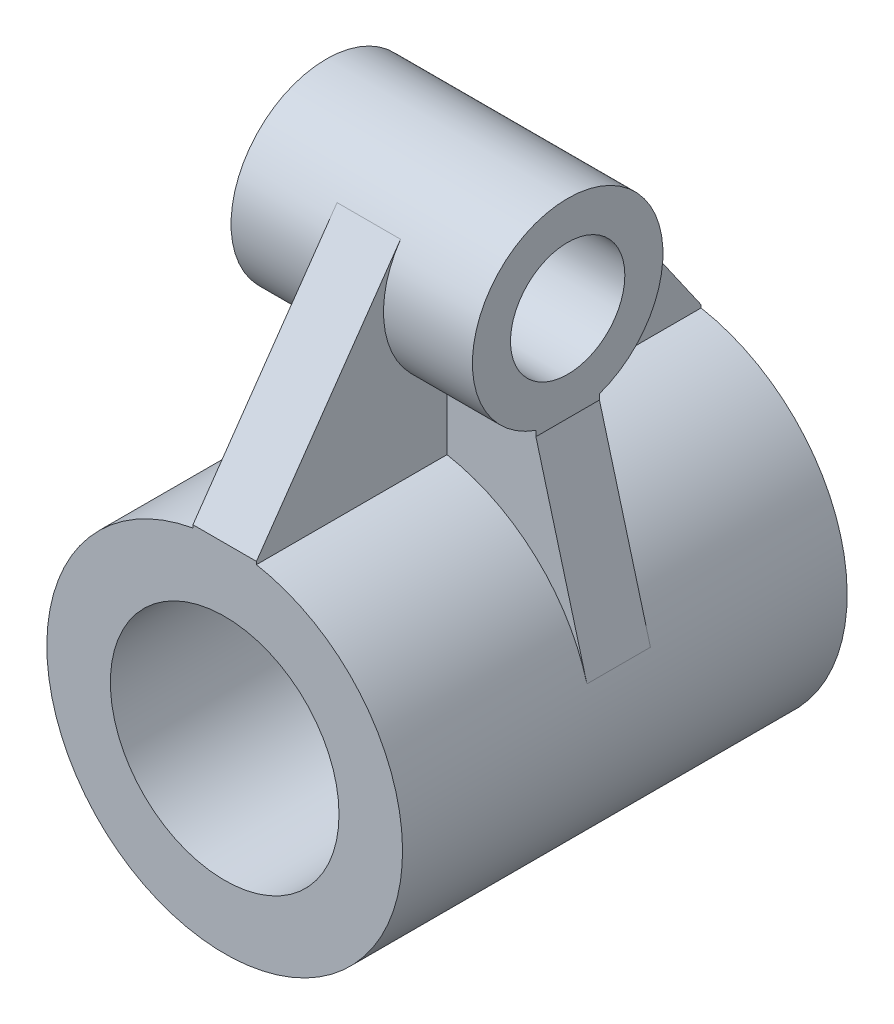
ISO-10303-21;
HEADER;
FILE_DESCRIPTION(('STEP AP214'),'2;1');
FILE_NAME('part.step','',(''),(''),'','','');
FILE_SCHEMA(('AUTOMOTIVE_DESIGN { 1 0 10303 214 1 1 1 1 }'));
ENDSEC;
DATA;
#1=APPLICATION_CONTEXT('core data for automotive mechanical design processes');
#2=APPLICATION_PROTOCOL_DEFINITION('international standard','automotive_design',2000,#1);
#3=PRODUCT_CONTEXT('',#1,'mechanical');
#4=PRODUCT('Part','Part','',(#3));
#5=PRODUCT_RELATED_PRODUCT_CATEGORY('part','',(#4));
#6=PRODUCT_DEFINITION_FORMATION('','',#4);
#7=PRODUCT_DEFINITION_CONTEXT('part definition',#1,'design');
#8=PRODUCT_DEFINITION('design','',#6,#7);
#9=PRODUCT_DEFINITION_SHAPE('','',#8);
#10=(LENGTH_UNIT() NAMED_UNIT(*) SI_UNIT(.MILLI.,.METRE.));
#11=(NAMED_UNIT(*) PLANE_ANGLE_UNIT() SI_UNIT($,.RADIAN.));
#12=(NAMED_UNIT(*) SI_UNIT($,.STERADIAN.) SOLID_ANGLE_UNIT());
#13=UNCERTAINTY_MEASURE_WITH_UNIT(LENGTH_MEASURE(1.E-05),#10,'distance_accuracy_value','');
#14=(GEOMETRIC_REPRESENTATION_CONTEXT(3) GLOBAL_UNCERTAINTY_ASSIGNED_CONTEXT((#13)) GLOBAL_UNIT_ASSIGNED_CONTEXT((#10,
#11,#12)) REPRESENTATION_CONTEXT('',''));
#15=CARTESIAN_POINT('',(0.,0.,0.));
#16=DIRECTION('',(0.,0.,1.));
#17=DIRECTION('',(1.,0.,0.));
#18=AXIS2_PLACEMENT_3D('',#15,#16,#17);
#19=CARTESIAN_POINT('',(0.,0.,17.5));
#20=DIRECTION('',(0.,0.,-1.));
#21=DIRECTION('',(-1.,0.,0.));
#22=AXIS2_PLACEMENT_3D('',#19,#20,#21);
#23=CYLINDRICAL_SURFACE('',#22,14.);
#24=CARTESIAN_POINT('',(0.,0.,2.5));
#25=DIRECTION('',(0.,0.,-1.));
#26=DIRECTION('',(1.,0.,0.));
#27=AXIS2_PLACEMENT_3D('',#24,#25,#26);
#28=CIRCLE('',#27,14.);
#29=CARTESIAN_POINT('',(-13.5145575336428,3.65468667191318,2.5));
#30=VERTEX_POINT('',#29);
#31=CARTESIAN_POINT('',(-2.5,13.7749773139559,2.5));
#32=VERTEX_POINT('',#31);
#33=EDGE_CURVE('E182',#30,#32,#28,.T.);
#34=ORIENTED_EDGE('',*,*,#33,.F.);
#35=DIRECTION('',(0.,0.,-1.));
#36=VECTOR('',#35,1.);
#37=CARTESIAN_POINT('',(-13.5145575336428,3.65468667191318,2.5));
#38=LINE('',#37,#36);
#39=CARTESIAN_POINT('',(-13.5145575336428,3.65468667191318,-2.5));
#40=VERTEX_POINT('',#39);
#41=EDGE_CURVE('E178',#30,#40,#38,.T.);
#42=ORIENTED_EDGE('',*,*,#41,.T.);
#43=CARTESIAN_POINT('',(0.,0.,-2.5));
#44=DIRECTION('',(0.,0.,-1.));
#45=DIRECTION('',(1.,0.,0.));
#46=AXIS2_PLACEMENT_3D('',#43,#44,#45);
#47=CIRCLE('',#46,14.);
#48=CARTESIAN_POINT('',(-2.5,13.7749773139559,-2.5));
#49=VERTEX_POINT('',#48);
#50=EDGE_CURVE('E190',#40,#49,#47,.T.);
#51=ORIENTED_EDGE('',*,*,#50,.T.);
#52=DIRECTION('',(0.,0.,-1.));
#53=VECTOR('',#52,1.);
#54=CARTESIAN_POINT('',(-2.5,13.7749773139559,17.5));
#55=LINE('',#54,#53);
#56=CARTESIAN_POINT('',(-2.5,13.7749773139559,-17.5));
#57=VERTEX_POINT('',#56);
#58=EDGE_CURVE('E11',#57,#49,#55,.F.);
#59=ORIENTED_EDGE('',*,*,#58,.F.);
#60=CARTESIAN_POINT('',(0.,0.,-17.5));
#61=DIRECTION('',(0.,0.,1.));
#62=DIRECTION('',(1.,0.,0.));
#63=AXIS2_PLACEMENT_3D('',#60,#61,#62);
#64=CIRCLE('',#63,14.);
#65=CARTESIAN_POINT('',(2.5,13.7749773139559,-17.5));
#66=VERTEX_POINT('',#65);
#67=EDGE_CURVE('E272',#57,#66,#64,.T.);
#68=ORIENTED_EDGE('',*,*,#67,.T.);
#69=DIRECTION('',(0.,0.,-1.));
#70=VECTOR('',#69,1.);
#71=CARTESIAN_POINT('',(2.5,13.7749773139559,17.5));
#72=LINE('',#71,#70);
#73=CARTESIAN_POINT('',(2.5,13.7749773139559,-2.5));
#74=VERTEX_POINT('',#73);
#75=EDGE_CURVE('E280',#74,#66,#72,.T.);
#76=ORIENTED_EDGE('',*,*,#75,.F.);
#77=CARTESIAN_POINT('',(13.5145575336428,3.65468667191318,-2.5));
#78=VERTEX_POINT('',#77);
#79=EDGE_CURVE('E59',#74,#78,#47,.T.);
#80=ORIENTED_EDGE('',*,*,#79,.T.);
#81=DIRECTION('',(0.,0.,-1.));
#82=VECTOR('',#81,1.);
#83=CARTESIAN_POINT('',(13.5145575336428,3.65468667191318,2.5));
#84=LINE('',#83,#82);
#85=CARTESIAN_POINT('',(13.5145575336428,3.65468667191318,2.5));
#86=VERTEX_POINT('',#85);
#87=EDGE_CURVE('E52',#86,#78,#84,.T.);
#88=ORIENTED_EDGE('',*,*,#87,.F.);
#89=CARTESIAN_POINT('',(2.5,13.7749773139559,2.5));
#90=VERTEX_POINT('',#89);
#91=EDGE_CURVE('E191',#90,#86,#28,.T.);
#92=ORIENTED_EDGE('',*,*,#91,.F.);
#93=CARTESIAN_POINT('',(2.5,13.7749773139559,17.5));
#94=VERTEX_POINT('',#93);
#95=EDGE_CURVE('E276',#94,#90,#72,.T.);
#96=ORIENTED_EDGE('',*,*,#95,.F.);
#97=CARTESIAN_POINT('',(0.,0.,17.5));
#98=DIRECTION('',(0.,0.,1.));
#99=DIRECTION('',(1.,0.,0.));
#100=AXIS2_PLACEMENT_3D('',#97,#98,#99);
#101=CIRCLE('',#100,14.);
#102=CARTESIAN_POINT('',(-2.5,13.7749773139559,17.5));
#103=VERTEX_POINT('',#102);
#104=EDGE_CURVE('E274',#103,#94,#101,.T.);
#105=ORIENTED_EDGE('',*,*,#104,.F.);
#106=EDGE_CURVE('E46',#32,#103,#55,.F.);
#107=ORIENTED_EDGE('',*,*,#106,.F.);
#108=EDGE_LOOP('',(#34,#42,#51,#59,#68,#76,#80,#88,#92,#96,#105,#107));
#109=FACE_BOUND('',#108,.T.);
#110=ADVANCED_FACE('F39',(#109),#23,.T.);
#111=CARTESIAN_POINT('',(-2.5,11.,17.5));
#112=DIRECTION('',(1.,0.,0.));
#113=DIRECTION('',(0.,0.,-1.));
#114=AXIS2_PLACEMENT_3D('',#111,#112,#113);
#115=PLANE('',#114);
#116=ORIENTED_EDGE('',*,*,#58,.T.);
#117=DIRECTION('',(0.,-1.,0.));
#118=VECTOR('',#117,1.);
#119=CARTESIAN_POINT('',(-2.5,26.,-2.5));
#120=LINE('',#119,#118);
#121=CARTESIAN_POINT('',(-2.5,18.9289321881345,-2.5));
#122=VERTEX_POINT('',#121);
#123=EDGE_CURVE('E243',#122,#49,#120,.T.);
#124=ORIENTED_EDGE('',*,*,#123,.F.);
#125=CARTESIAN_POINT('',(-2.5,26.,0.));
#126=DIRECTION('',(-1.,0.,0.));
#127=DIRECTION('',(0.,0.,-1.));
#128=AXIS2_PLACEMENT_3D('',#125,#126,#127);
#129=CIRCLE('',#128,7.5);
#130=CARTESIAN_POINT('',(-2.5,30.2870363418498,-6.15396777726847));
#131=VERTEX_POINT('',#130);
#132=EDGE_CURVE('E223',#131,#122,#129,.T.);
#133=ORIENTED_EDGE('',*,*,#132,.F.);
#134=DIRECTION('',(0.,0.820529036969129,0.57160484557998));
#135=VECTOR('',#134,1.);
#136=CARTESIAN_POINT('',(-2.5,14.,-17.5));
#137=LINE('',#136,#135);
#138=CARTESIAN_POINT('',(-2.5,14.,-17.5));
#139=VERTEX_POINT('',#138);
#140=EDGE_CURVE('E219',#139,#131,#137,.T.);
#141=ORIENTED_EDGE('',*,*,#140,.F.);
#142=DIRECTION('',(0.,1.,0.));
#143=VECTOR('',#142,1.);
#144=CARTESIAN_POINT('',(-2.5,11.,-17.5));
#145=LINE('',#144,#143);
#146=EDGE_CURVE('E264',#57,#139,#145,.T.);
#147=ORIENTED_EDGE('',*,*,#146,.F.);
#148=EDGE_LOOP('',(#116,#124,#133,#141,#147));
#149=FACE_BOUND('',#148,.T.);
#150=ADVANCED_FACE('F350',(#149),#115,.F.);
#151=DIRECTION('',(0.,1.,0.));
#152=VECTOR('',#151,1.);
#153=CARTESIAN_POINT('',(-2.5,11.,2.5));
#154=LINE('',#153,#152);
#155=CARTESIAN_POINT('',(-2.5,18.9289321881345,2.5));
#156=VERTEX_POINT('',#155);
#157=EDGE_CURVE('E252',#32,#156,#154,.T.);
#158=ORIENTED_EDGE('',*,*,#157,.F.);
#159=ORIENTED_EDGE('',*,*,#106,.T.);
#160=DIRECTION('',(0.,1.,0.));
#161=VECTOR('',#160,1.);
#162=CARTESIAN_POINT('',(-2.5,11.,17.5));
#163=LINE('',#162,#161);
#164=CARTESIAN_POINT('',(-2.5,14.,17.5));
#165=VERTEX_POINT('',#164);
#166=EDGE_CURVE('E259',#103,#165,#163,.T.);
#167=ORIENTED_EDGE('',*,*,#166,.T.);
#168=DIRECTION('',(0.,-0.820529036969129,0.57160484557998));
#169=VECTOR('',#168,1.);
#170=CARTESIAN_POINT('',(-2.5,14.,17.5));
#171=LINE('',#170,#169);
#172=CARTESIAN_POINT('',(-2.5,30.2870363418499,6.15396777726847));
#173=VERTEX_POINT('',#172);
#174=EDGE_CURVE('E215',#173,#165,#171,.T.);
#175=ORIENTED_EDGE('',*,*,#174,.F.);
#176=EDGE_CURVE('E225',#156,#173,#129,.T.);
#177=ORIENTED_EDGE('',*,*,#176,.F.);
#178=EDGE_LOOP('',(#158,#159,#167,#175,#177));
#179=FACE_BOUND('',#178,.T.);
#180=ADVANCED_FACE('F316',(#179),#115,.F.);
#181=CARTESIAN_POINT('',(2.5,11.,17.5));
#182=DIRECTION('',(-1.,0.,0.));
#183=DIRECTION('',(0.,0.,1.));
#184=AXIS2_PLACEMENT_3D('',#181,#182,#183);
#185=PLANE('',#184);
#186=DIRECTION('',(0.,-1.,0.));
#187=VECTOR('',#186,1.);
#188=CARTESIAN_POINT('',(2.5,11.,2.5));
#189=LINE('',#188,#187);
#190=CARTESIAN_POINT('',(2.5,18.9289321881345,2.5));
#191=VERTEX_POINT('',#190);
#192=EDGE_CURVE('E247',#191,#90,#189,.T.);
#193=ORIENTED_EDGE('',*,*,#192,.F.);
#194=CARTESIAN_POINT('',(2.5,26.,0.));
#195=DIRECTION('',(-1.,0.,0.));
#196=DIRECTION('',(0.,0.,-1.));
#197=AXIS2_PLACEMENT_3D('',#194,#195,#196);
#198=CIRCLE('',#197,7.5);
#199=CARTESIAN_POINT('',(2.5,30.2870363418499,6.15396777726847));
#200=VERTEX_POINT('',#199);
#201=EDGE_CURVE('E212',#191,#200,#198,.T.);
#202=ORIENTED_EDGE('',*,*,#201,.T.);
#203=DIRECTION('',(0.,-0.820529036969129,0.57160484557998));
#204=VECTOR('',#203,1.);
#205=CARTESIAN_POINT('',(2.5,14.,17.5));
#206=LINE('',#205,#204);
#207=CARTESIAN_POINT('',(2.5,14.,17.5));
#208=VERTEX_POINT('',#207);
#209=EDGE_CURVE('E216',#200,#208,#206,.T.);
#210=ORIENTED_EDGE('',*,*,#209,.T.);
#211=DIRECTION('',(0.,1.,0.));
#212=VECTOR('',#211,1.);
#213=CARTESIAN_POINT('',(2.5,11.,17.5));
#214=LINE('',#213,#212);
#215=EDGE_CURVE('E261',#94,#208,#214,.T.);
#216=ORIENTED_EDGE('',*,*,#215,.F.);
#217=ORIENTED_EDGE('',*,*,#95,.T.);
#218=EDGE_LOOP('',(#193,#202,#210,#216,#217));
#219=FACE_BOUND('',#218,.T.);
#220=ADVANCED_FACE('F328',(#219),#185,.F.);
#221=DIRECTION('',(0.,1.,0.));
#222=VECTOR('',#221,1.);
#223=CARTESIAN_POINT('',(2.5,11.,-2.5));
#224=LINE('',#223,#222);
#225=CARTESIAN_POINT('',(2.5,18.9289321881345,-2.5));
#226=VERTEX_POINT('',#225);
#227=EDGE_CURVE('E246',#74,#226,#224,.T.);
#228=ORIENTED_EDGE('',*,*,#227,.F.);
#229=ORIENTED_EDGE('',*,*,#75,.T.);
#230=DIRECTION('',(0.,1.,0.));
#231=VECTOR('',#230,1.);
#232=CARTESIAN_POINT('',(2.5,11.,-17.5));
#233=LINE('',#232,#231);
#234=CARTESIAN_POINT('',(2.5,14.,-17.5));
#235=VERTEX_POINT('',#234);
#236=EDGE_CURVE('E263',#66,#235,#233,.T.);
#237=ORIENTED_EDGE('',*,*,#236,.T.);
#238=DIRECTION('',(0.,0.820529036969129,0.57160484557998));
#239=VECTOR('',#238,1.);
#240=CARTESIAN_POINT('',(2.5,14.,-17.5));
#241=LINE('',#240,#239);
#242=CARTESIAN_POINT('',(2.5,30.2870363418498,-6.15396777726847));
#243=VERTEX_POINT('',#242);
#244=EDGE_CURVE('E206',#235,#243,#241,.T.);
#245=ORIENTED_EDGE('',*,*,#244,.T.);
#246=EDGE_CURVE('E214',#243,#226,#198,.T.);
#247=ORIENTED_EDGE('',*,*,#246,.T.);
#248=EDGE_LOOP('',(#228,#229,#237,#245,#247));
#249=FACE_BOUND('',#248,.T.);
#250=ADVANCED_FACE('F282',(#249),#185,.F.);
#251=CARTESIAN_POINT('',(0.,0.,17.5));
#252=DIRECTION('',(0.,0.,1.));
#253=DIRECTION('',(1.,0.,0.));
#254=AXIS2_PLACEMENT_3D('',#251,#252,#253);
#255=PLANE('',#254);
#256=ORIENTED_EDGE('',*,*,#104,.T.);
#257=ORIENTED_EDGE('',*,*,#215,.T.);
#258=DIRECTION('',(-1.,0.,0.));
#259=VECTOR('',#258,1.);
#260=CARTESIAN_POINT('',(-2.5,14.,17.5));
#261=LINE('',#260,#259);
#262=EDGE_CURVE('E257',#208,#165,#261,.T.);
#263=ORIENTED_EDGE('',*,*,#262,.T.);
#264=ORIENTED_EDGE('',*,*,#166,.F.);
#265=EDGE_LOOP('',(#256,#257,#263,#264));
#266=FACE_BOUND('',#265,.T.);
#267=CARTESIAN_POINT('',(0.,0.,17.5));
#268=DIRECTION('',(0.,0.,1.));
#269=DIRECTION('',(1.,0.,0.));
#270=AXIS2_PLACEMENT_3D('',#267,#268,#269);
#271=CIRCLE('',#270,9.);
#272=CARTESIAN_POINT('',(9.,0.,17.5));
#273=VERTEX_POINT('',#272);
#274=EDGE_CURVE('E270',#273,#273,#271,.T.);
#275=ORIENTED_EDGE('',*,*,#274,.F.);
#276=EDGE_LOOP('',(#275));
#277=FACE_BOUND('',#276,.T.);
#278=ADVANCED_FACE('F329',(#266,#277),#255,.T.);
#279=CARTESIAN_POINT('',(0.,0.,-17.5));
#280=DIRECTION('',(0.,0.,1.));
#281=DIRECTION('',(1.,0.,0.));
#282=AXIS2_PLACEMENT_3D('',#279,#280,#281);
#283=PLANE('',#282);
#284=ORIENTED_EDGE('',*,*,#146,.T.);
#285=DIRECTION('',(1.,0.,0.));
#286=VECTOR('',#285,1.);
#287=CARTESIAN_POINT('',(-2.5,14.,-17.5));
#288=LINE('',#287,#286);
#289=EDGE_CURVE('E254',#139,#235,#288,.T.);
#290=ORIENTED_EDGE('',*,*,#289,.T.);
#291=ORIENTED_EDGE('',*,*,#236,.F.);
#292=ORIENTED_EDGE('',*,*,#67,.F.);
#293=EDGE_LOOP('',(#284,#290,#291,#292));
#294=FACE_BOUND('',#293,.T.);
#295=CARTESIAN_POINT('',(0.,0.,-17.5));
#296=DIRECTION('',(0.,0.,1.));
#297=DIRECTION('',(1.,0.,0.));
#298=AXIS2_PLACEMENT_3D('',#295,#296,#297);
#299=CIRCLE('',#298,9.);
#300=CARTESIAN_POINT('',(9.,0.,-17.5));
#301=VERTEX_POINT('',#300);
#302=EDGE_CURVE('E266',#301,#301,#299,.T.);
#303=ORIENTED_EDGE('',*,*,#302,.T.);
#304=EDGE_LOOP('',(#303));
#305=FACE_BOUND('',#304,.T.);
#306=ADVANCED_FACE('F288',(#294,#305),#283,.F.);
#307=CARTESIAN_POINT('',(0.,0.,17.5));
#308=DIRECTION('',(0.,0.,-1.));
#309=DIRECTION('',(-1.,0.,0.));
#310=AXIS2_PLACEMENT_3D('',#307,#308,#309);
#311=CYLINDRICAL_SURFACE('',#310,9.);
#312=ORIENTED_EDGE('',*,*,#274,.T.);
#313=EDGE_LOOP('',(#312));
#314=FACE_BOUND('',#313,.T.);
#315=ORIENTED_EDGE('',*,*,#302,.F.);
#316=EDGE_LOOP('',(#315));
#317=FACE_BOUND('',#316,.T.);
#318=ADVANCED_FACE('F337',(#314,#317),#311,.F.);
#319=CARTESIAN_POINT('',(-9.5,21.5,-2.5));
#320=DIRECTION('',(0.,0.,1.));
#321=DIRECTION('',(1.,0.,0.));
#322=AXIS2_PLACEMENT_3D('',#319,#320,#321);
#323=PLANE('',#322);
#324=ORIENTED_EDGE('',*,*,#123,.T.);
#325=ORIENTED_EDGE('',*,*,#50,.F.);
#326=DIRECTION('',(-0.261049047993799,-0.96532553811734,0.));
#327=VECTOR('',#326,1.);
#328=CARTESIAN_POINT('',(-13.5145575336428,3.65468667191318,-2.5));
#329=LINE('',#328,#327);
#330=CARTESIAN_POINT('',(-9.5,18.5,-2.5));
#331=VERTEX_POINT('',#330);
#332=EDGE_CURVE('E194',#331,#40,#329,.T.);
#333=ORIENTED_EDGE('',*,*,#332,.F.);
#334=DIRECTION('',(0.,-1.,0.));
#335=VECTOR('',#334,1.);
#336=CARTESIAN_POINT('',(-9.5,21.5,-2.5));
#337=LINE('',#336,#335);
#338=CARTESIAN_POINT('',(-9.5,18.9289321881345,-2.5));
#339=VERTEX_POINT('',#338);
#340=EDGE_CURVE('E171',#339,#331,#337,.T.);
#341=ORIENTED_EDGE('',*,*,#340,.F.);
#342=DIRECTION('',(-1.,0.,0.));
#343=VECTOR('',#342,1.);
#344=CARTESIAN_POINT('',(9.5,18.9289321881345,-2.5));
#345=LINE('',#344,#343);
#346=EDGE_CURVE('E161',#339,#122,#345,.F.);
#347=ORIENTED_EDGE('',*,*,#346,.T.);
#348=EDGE_LOOP('',(#324,#325,#333,#341,#347));
#349=FACE_BOUND('',#348,.T.);
#350=ADVANCED_FACE('F339',(#349),#323,.F.);
#351=CARTESIAN_POINT('',(-9.5,21.5,2.5));
#352=DIRECTION('',(0.,0.,-1.));
#353=DIRECTION('',(-1.,0.,0.));
#354=AXIS2_PLACEMENT_3D('',#351,#352,#353);
#355=PLANE('',#354);
#356=ORIENTED_EDGE('',*,*,#33,.T.);
#357=ORIENTED_EDGE('',*,*,#157,.T.);
#358=DIRECTION('',(-1.,0.,0.));
#359=VECTOR('',#358,1.);
#360=CARTESIAN_POINT('',(9.5,18.9289321881345,2.5));
#361=LINE('',#360,#359);
#362=CARTESIAN_POINT('',(-9.5,18.9289321881345,2.5));
#363=VERTEX_POINT('',#362);
#364=EDGE_CURVE('E157',#156,#363,#361,.T.);
#365=ORIENTED_EDGE('',*,*,#364,.T.);
#366=DIRECTION('',(0.,-1.,0.));
#367=VECTOR('',#366,1.);
#368=CARTESIAN_POINT('',(-9.5,21.5,2.5));
#369=LINE('',#368,#367);
#370=CARTESIAN_POINT('',(-9.5,18.5,2.5));
#371=VERTEX_POINT('',#370);
#372=EDGE_CURVE('E155',#363,#371,#369,.T.);
#373=ORIENTED_EDGE('',*,*,#372,.T.);
#374=DIRECTION('',(-0.261049047993799,-0.96532553811734,0.));
#375=VECTOR('',#374,1.);
#376=CARTESIAN_POINT('',(-13.5145575336428,3.65468667191318,2.5));
#377=LINE('',#376,#375);
#378=EDGE_CURVE('E156',#371,#30,#377,.T.);
#379=ORIENTED_EDGE('',*,*,#378,.T.);
#380=EDGE_LOOP('',(#356,#357,#365,#373,#379));
#381=FACE_BOUND('',#380,.T.);
#382=ADVANCED_FACE('F154',(#381),#355,.F.);
#383=CARTESIAN_POINT('',(9.5,18.9289321881345,2.5));
#384=VERTEX_POINT('',#383);
#385=EDGE_CURVE('E210',#384,#191,#361,.T.);
#386=ORIENTED_EDGE('',*,*,#385,.T.);
#387=ORIENTED_EDGE('',*,*,#192,.T.);
#388=ORIENTED_EDGE('',*,*,#91,.T.);
#389=DIRECTION('',(-0.261049047993799,0.96532553811734,0.));
#390=VECTOR('',#389,1.);
#391=CARTESIAN_POINT('',(9.5,18.5,2.5));
#392=LINE('',#391,#390);
#393=CARTESIAN_POINT('',(9.5,18.5,2.5));
#394=VERTEX_POINT('',#393);
#395=EDGE_CURVE('E177',#86,#394,#392,.T.);
#396=ORIENTED_EDGE('',*,*,#395,.T.);
#397=DIRECTION('',(0.,-1.,0.));
#398=VECTOR('',#397,1.);
#399=CARTESIAN_POINT('',(9.5,21.5,2.5));
#400=LINE('',#399,#398);
#401=EDGE_CURVE('E165',#384,#394,#400,.T.);
#402=ORIENTED_EDGE('',*,*,#401,.F.);
#403=EDGE_LOOP('',(#386,#387,#388,#396,#402));
#404=FACE_BOUND('',#403,.T.);
#405=ADVANCED_FACE('F313',(#404),#355,.F.);
#406=ORIENTED_EDGE('',*,*,#79,.F.);
#407=ORIENTED_EDGE('',*,*,#227,.T.);
#408=CARTESIAN_POINT('',(9.5,18.9289321881345,-2.5));
#409=VERTEX_POINT('',#408);
#410=EDGE_CURVE('E202',#226,#409,#345,.F.);
#411=ORIENTED_EDGE('',*,*,#410,.T.);
#412=DIRECTION('',(0.,-1.,0.));
#413=VECTOR('',#412,1.);
#414=CARTESIAN_POINT('',(9.5,21.5,-2.5));
#415=LINE('',#414,#413);
#416=CARTESIAN_POINT('',(9.5,18.5,-2.5));
#417=VERTEX_POINT('',#416);
#418=EDGE_CURVE('E197',#409,#417,#415,.T.);
#419=ORIENTED_EDGE('',*,*,#418,.T.);
#420=DIRECTION('',(-0.261049047993799,0.96532553811734,0.));
#421=VECTOR('',#420,1.);
#422=CARTESIAN_POINT('',(9.5,18.5,-2.5));
#423=LINE('',#422,#421);
#424=EDGE_CURVE('E188',#78,#417,#423,.T.);
#425=ORIENTED_EDGE('',*,*,#424,.F.);
#426=EDGE_LOOP('',(#406,#407,#411,#419,#425));
#427=FACE_BOUND('',#426,.T.);
#428=ADVANCED_FACE('F302',(#427),#323,.F.);
#429=CARTESIAN_POINT('',(9.5,26.,0.));
#430=DIRECTION('',(-1.,0.,0.));
#431=DIRECTION('',(0.,0.,1.));
#432=AXIS2_PLACEMENT_3D('',#429,#430,#431);
#433=CYLINDRICAL_SURFACE('',#432,7.5);
#434=ORIENTED_EDGE('',*,*,#385,.F.);
#435=CARTESIAN_POINT('',(9.5,26.,0.));
#436=DIRECTION('',(1.,0.,0.));
#437=DIRECTION('',(0.,0.,-1.));
#438=AXIS2_PLACEMENT_3D('',#435,#436,#437);
#439=CIRCLE('',#438,7.5);
#440=EDGE_CURVE('E239',#409,#384,#439,.T.);
#441=ORIENTED_EDGE('',*,*,#440,.F.);
#442=ORIENTED_EDGE('',*,*,#410,.F.);
#443=ORIENTED_EDGE('',*,*,#246,.F.);
#444=DIRECTION('',(-1.,0.,0.));
#445=VECTOR('',#444,1.);
#446=CARTESIAN_POINT('',(2.5,30.2870363418498,-6.15396777726847));
#447=LINE('',#446,#445);
#448=EDGE_CURVE('E233',#243,#131,#447,.T.);
#449=ORIENTED_EDGE('',*,*,#448,.T.);
#450=ORIENTED_EDGE('',*,*,#132,.T.);
#451=ORIENTED_EDGE('',*,*,#346,.F.);
#452=CARTESIAN_POINT('',(-9.5,26.,0.));
#453=DIRECTION('',(1.,0.,0.));
#454=DIRECTION('',(0.,0.,-1.));
#455=AXIS2_PLACEMENT_3D('',#452,#453,#454);
#456=CIRCLE('',#455,7.5);
#457=EDGE_CURVE('E240',#339,#363,#456,.T.);
#458=ORIENTED_EDGE('',*,*,#457,.T.);
#459=ORIENTED_EDGE('',*,*,#364,.F.);
#460=ORIENTED_EDGE('',*,*,#176,.T.);
#461=DIRECTION('',(-1.,0.,0.));
#462=VECTOR('',#461,1.);
#463=CARTESIAN_POINT('',(2.5,30.2870363418499,6.15396777726847));
#464=LINE('',#463,#462);
#465=EDGE_CURVE('E217',#200,#173,#464,.T.);
#466=ORIENTED_EDGE('',*,*,#465,.F.);
#467=ORIENTED_EDGE('',*,*,#201,.F.);
#468=EDGE_LOOP('',(#434,#441,#442,#443,#449,#450,#451,#458,#459,#460,#466,#467));
#469=FACE_BOUND('',#468,.T.);
#470=ADVANCED_FACE('F297',(#469),#433,.T.);
#471=CARTESIAN_POINT('',(9.5,26.,0.));
#472=DIRECTION('',(1.,0.,0.));
#473=DIRECTION('',(0.,0.,-1.));
#474=AXIS2_PLACEMENT_3D('',#471,#472,#473);
#475=PLANE('',#474);
#476=ORIENTED_EDGE('',*,*,#440,.T.);
#477=ORIENTED_EDGE('',*,*,#401,.T.);
#478=DIRECTION('',(0.,0.,-1.));
#479=VECTOR('',#478,1.);
#480=CARTESIAN_POINT('',(9.5,18.5,-2.5));
#481=LINE('',#480,#479);
#482=EDGE_CURVE('E174',#394,#417,#481,.T.);
#483=ORIENTED_EDGE('',*,*,#482,.T.);
#484=ORIENTED_EDGE('',*,*,#418,.F.);
#485=EDGE_LOOP('',(#476,#477,#483,#484));
#486=FACE_BOUND('',#485,.T.);
#487=CARTESIAN_POINT('',(9.5,26.,0.));
#488=DIRECTION('',(1.,0.,0.));
#489=DIRECTION('',(0.,0.,-1.));
#490=AXIS2_PLACEMENT_3D('',#487,#488,#489);
#491=CIRCLE('',#490,4.5);
#492=CARTESIAN_POINT('',(9.5,26.,-4.5));
#493=VERTEX_POINT('',#492);
#494=EDGE_CURVE('E234',#493,#493,#491,.T.);
#495=ORIENTED_EDGE('',*,*,#494,.F.);
#496=EDGE_LOOP('',(#495));
#497=FACE_BOUND('',#496,.T.);
#498=ADVANCED_FACE('F306',(#486,#497),#475,.T.);
#499=CARTESIAN_POINT('',(-9.5,26.,0.));
#500=DIRECTION('',(1.,0.,0.));
#501=DIRECTION('',(0.,0.,-1.));
#502=AXIS2_PLACEMENT_3D('',#499,#500,#501);
#503=PLANE('',#502);
#504=ORIENTED_EDGE('',*,*,#340,.T.);
#505=DIRECTION('',(0.,0.,1.));
#506=VECTOR('',#505,1.);
#507=CARTESIAN_POINT('',(-9.5,18.5,-2.5));
#508=LINE('',#507,#506);
#509=EDGE_CURVE('E170',#331,#371,#508,.T.);
#510=ORIENTED_EDGE('',*,*,#509,.T.);
#511=ORIENTED_EDGE('',*,*,#372,.F.);
#512=ORIENTED_EDGE('',*,*,#457,.F.);
#513=EDGE_LOOP('',(#504,#510,#511,#512));
#514=FACE_BOUND('',#513,.T.);
#515=CARTESIAN_POINT('',(-9.5,26.,0.));
#516=DIRECTION('',(1.,0.,0.));
#517=DIRECTION('',(0.,0.,-1.));
#518=AXIS2_PLACEMENT_3D('',#515,#516,#517);
#519=CIRCLE('',#518,4.5);
#520=CARTESIAN_POINT('',(-9.5,26.,-4.5));
#521=VERTEX_POINT('',#520);
#522=EDGE_CURVE('E231',#521,#521,#519,.T.);
#523=ORIENTED_EDGE('',*,*,#522,.T.);
#524=EDGE_LOOP('',(#523));
#525=FACE_BOUND('',#524,.T.);
#526=ADVANCED_FACE('F166',(#514,#525),#503,.F.);
#527=CARTESIAN_POINT('',(9.5,26.,0.));
#528=DIRECTION('',(-1.,0.,0.));
#529=DIRECTION('',(0.,0.,1.));
#530=AXIS2_PLACEMENT_3D('',#527,#528,#529);
#531=CYLINDRICAL_SURFACE('',#530,4.5);
#532=ORIENTED_EDGE('',*,*,#522,.F.);
#533=EDGE_LOOP('',(#532));
#534=FACE_BOUND('',#533,.T.);
#535=ORIENTED_EDGE('',*,*,#494,.T.);
#536=EDGE_LOOP('',(#535));
#537=FACE_BOUND('',#536,.T.);
#538=ADVANCED_FACE('F361',(#534,#537),#531,.F.);
#539=CARTESIAN_POINT('',(2.5,14.,-17.5));
#540=DIRECTION('',(0.,-0.57160484557998,0.820529036969129));
#541=DIRECTION('',(0.,-0.820529036969129,-0.571604845579981));
#542=AXIS2_PLACEMENT_3D('',#539,#540,#541);
#543=PLANE('',#542);
#544=ORIENTED_EDGE('',*,*,#140,.T.);
#545=ORIENTED_EDGE('',*,*,#448,.F.);
#546=ORIENTED_EDGE('',*,*,#244,.F.);
#547=ORIENTED_EDGE('',*,*,#289,.F.);
#548=EDGE_LOOP('',(#544,#545,#546,#547));
#549=FACE_BOUND('',#548,.T.);
#550=ADVANCED_FACE('F298',(#549),#543,.F.);
#551=CARTESIAN_POINT('',(2.5,14.,17.5));
#552=DIRECTION('',(0.,-0.57160484557998,-0.820529036969129));
#553=DIRECTION('',(0.,0.820529036969129,-0.571604845579981));
#554=AXIS2_PLACEMENT_3D('',#551,#552,#553);
#555=PLANE('',#554);
#556=ORIENTED_EDGE('',*,*,#174,.T.);
#557=ORIENTED_EDGE('',*,*,#262,.F.);
#558=ORIENTED_EDGE('',*,*,#209,.F.);
#559=ORIENTED_EDGE('',*,*,#465,.T.);
#560=EDGE_LOOP('',(#556,#557,#558,#559));
#561=FACE_BOUND('',#560,.T.);
#562=ADVANCED_FACE('F326',(#561),#555,.F.);
#563=CARTESIAN_POINT('',(9.5,18.5,2.5));
#564=DIRECTION('',(-0.96532553811734,-0.261049047993799,0.));
#565=DIRECTION('',(0.261049047993799,-0.96532553811734,0.));
#566=AXIS2_PLACEMENT_3D('',#563,#564,#565);
#567=PLANE('',#566);
#568=ORIENTED_EDGE('',*,*,#424,.T.);
#569=ORIENTED_EDGE('',*,*,#482,.F.);
#570=ORIENTED_EDGE('',*,*,#395,.F.);
#571=ORIENTED_EDGE('',*,*,#87,.T.);
#572=EDGE_LOOP('',(#568,#569,#570,#571));
#573=FACE_BOUND('',#572,.T.);
#574=ADVANCED_FACE('F311',(#573),#567,.F.);
#575=CARTESIAN_POINT('',(-13.5145575336428,3.65468667191318,2.5));
#576=DIRECTION('',(0.96532553811734,-0.261049047993799,0.));
#577=DIRECTION('',(0.261049047993799,0.96532553811734,0.));
#578=AXIS2_PLACEMENT_3D('',#575,#576,#577);
#579=PLANE('',#578);
#580=ORIENTED_EDGE('',*,*,#332,.T.);
#581=ORIENTED_EDGE('',*,*,#41,.F.);
#582=ORIENTED_EDGE('',*,*,#378,.F.);
#583=ORIENTED_EDGE('',*,*,#509,.F.);
#584=EDGE_LOOP('',(#580,#581,#582,#583));
#585=FACE_BOUND('',#584,.T.);
#586=ADVANCED_FACE('F180',(#585),#579,.F.);
#587=CLOSED_SHELL('',(#110,#150,#180,#220,#250,#278,#306,#318,#350,#382,#405,#428,#470,#498,
#526,#538,#550,#562,#574,#586));
#588=MANIFOLD_SOLID_BREP('B2',#587);
#589=ADVANCED_BREP_SHAPE_REPRESENTATION('',(#18,#588),#14);
#590=SHAPE_DEFINITION_REPRESENTATION(#9,#589);
ENDSEC;
END-ISO-10303-21;
